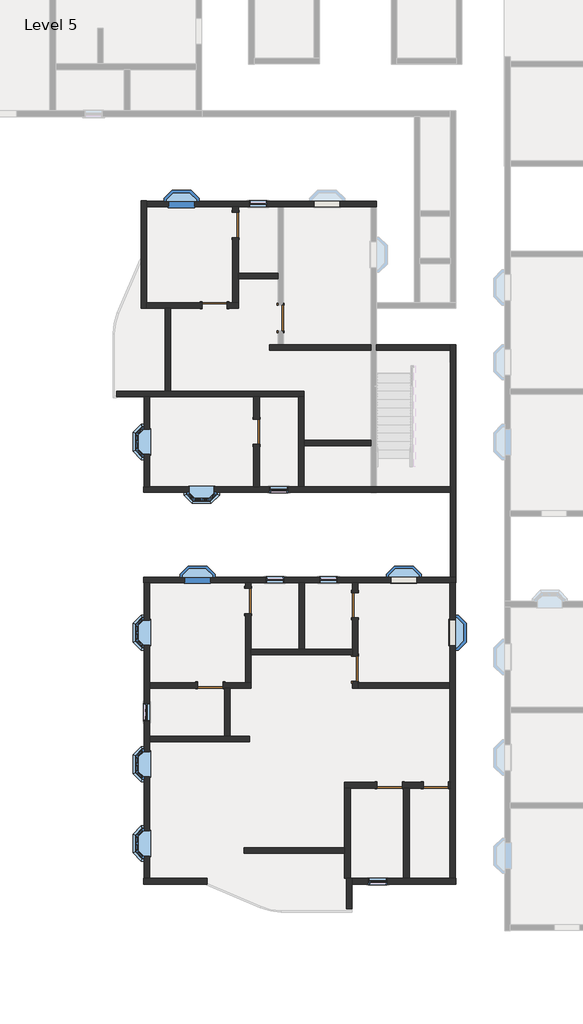
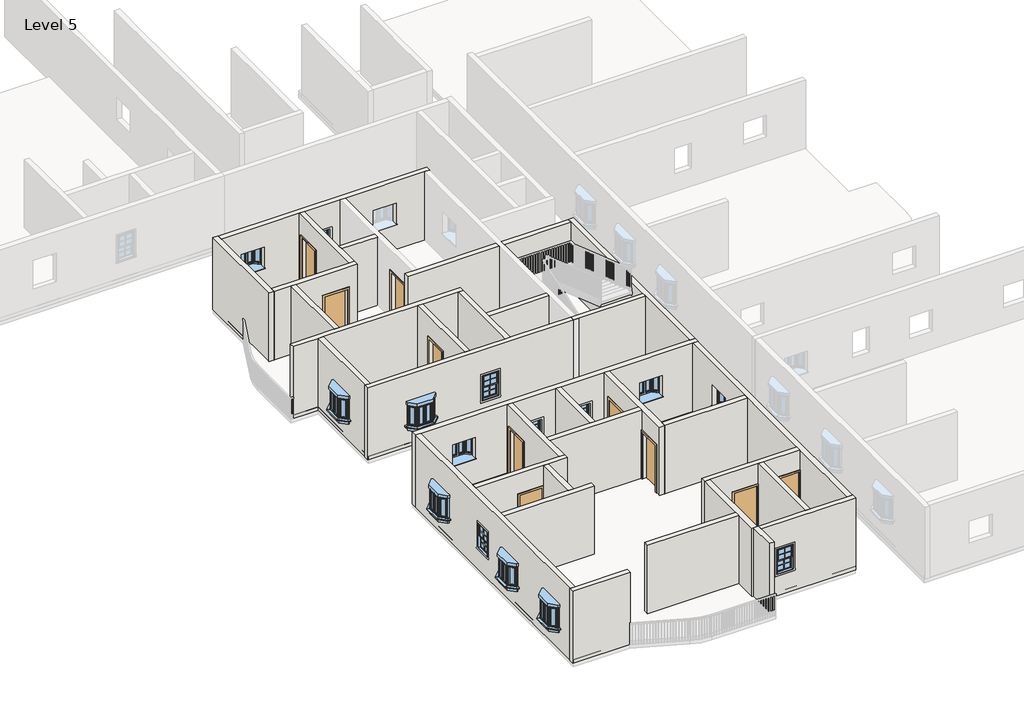
# One storey, part 1 of 14: 32 walls, 15 windows, 10 doors.
"""IFC4 building model written with IfcOpenShell, lengths in millimetres."""

from ifc_helpers import new_model, si_unit, frame, origin, place, context, project, spatial, polyline, outline, extrude, faceted_brep, transform, mapped, element, save
from components import door_54dd4da4, door_719f80de, window_910x910mm_67ef725a, window_8debb0fa

model = new_model("IFC4")

# Units and contexts
model_context = context("Model", 3, world=origin())
ifc_project = project(units=[si_unit("LENGTHUNIT", "METRE", prefix="MILLI")], contexts=[model_context])

# Site, building, storey
site = spatial("IfcSite", under=ifc_project)
building = spatial("IfcBuilding", under=site)
storey = spatial("IfcBuildingStorey", under=building, Name="Level 5", Elevation=12192.0)

# Doors
placement = place(None, origin())
door_shape = door_54dd4da4(model_context)
element("IfcDoor", 1, ObjectType="Single-Flush : 36\" x 84\"", at=placement, inside=storey, context=model_context, shape_type="MappedRepresentation", body=[
    mapped(door_shape, transform((-4626.037215, -17283.4916506, 12192.0), x_axis=(0.0, -1.0, 0.0), y_axis=(1.0, 0.0, 0.0), z_axis=(0.0, 0.0, 1.0))),
])
element("IfcDoor", 2, ObjectType="Single-Flush : 36\" x 84\"", at=placement, inside=storey, context=model_context, shape_type="MappedRepresentation", body=[
    mapped(door_shape, transform((-4626.037215, -14978.4416506, 12192.0), x_axis=(0.0, 1.0, 0.0), y_axis=(-1.0, 0.0, 0.0), z_axis=(0.0, 0.0, 1.0))),
])
element("IfcDoor", 3, ObjectType="Single-Flush : 36\" x 84\"", at=placement, inside=storey, context=model_context, shape_type="MappedRepresentation", body=[
    mapped(door_shape, transform((-9731.437215, -4100.8916506, 12192.0), x_axis=(1.0, 0.0, 0.0), y_axis=(0.0, 1.0, 0.0), z_axis=(0.0, 0.0, 1.0))),
])
element("IfcDoor", 4, ObjectType="Single-Flush : 36\" x 84\"", at=placement, inside=storey, context=model_context, shape_type="MappedRepresentation", body=[
    mapped(door_shape, transform((-7331.137215, -4558.0916506, 12192.0), x_axis=(0.0, -1.0, 0.0), y_axis=(1.0, 0.0, 0.0), z_axis=(0.0, 0.0, 1.0))),
])
door_2_shape = door_719f80de(model_context)
element("IfcDoor", 5, ObjectType="Single-Flush : 36\" x 84\"", at=placement, inside=storey, context=model_context, shape_type="MappedRepresentation", body=[
    mapped(door_2_shape, transform((-9883.837215, -17891.2072331, 12192.0), x_axis=(1.0, 0.0, 0.0), y_axis=(0.0, 1.0, 0.0), z_axis=(0.0, 0.0, 1.0))),
])
element("IfcDoor", 6, ObjectType="Single-Flush : 36\" x 84\"", at=placement, inside=storey, context=model_context, shape_type="MappedRepresentation", body=[
    mapped(door_2_shape, transform((-8512.237215, -14826.0416506, 12192.0), x_axis=(0.0, 1.0, 0.0), y_axis=(-1.0, 0.0, 0.0), z_axis=(0.0, 0.0, 1.0))),
])
element("IfcDoor", 7, ObjectType="Single-Flush : 36\" x 84\"", at=placement, inside=storey, context=model_context, shape_type="MappedRepresentation", body=[
    mapped(door_2_shape, transform((-8207.437215, -8691.9416506, 12192.0), x_axis=(0.0, 1.0, 0.0), y_axis=(-1.0, 0.0, 0.0), z_axis=(0.0, 0.0, 1.0))),
])
element("IfcDoor", 8, ObjectType="Single-Flush : 36\" x 84\"", at=placement, inside=storey, context=model_context, shape_type="MappedRepresentation", body=[
    mapped(door_2_shape, transform((-8969.437215, -1186.2416506, 12192.0), x_axis=(0.0, 1.0, 0.0), y_axis=(-1.0, 0.0, 0.0), z_axis=(0.0, 0.0, 1.0))),
])
element("IfcDoor", 9, ObjectType="Single-Flush : 36\" x 84\"", at=placement, inside=storey, context=model_context, shape_type="MappedRepresentation", body=[
    mapped(door_2_shape, transform((-3374.4891351, -21512.5916506, 12192.0), x_axis=(1.0, 0.0, 0.0), y_axis=(0.0, 1.0, 0.0), z_axis=(0.0, 0.0, 1.0))),
])
element("IfcDoor", 10, ObjectType="Single-Flush : 36\" x 84\"", at=placement, inside=storey, context=model_context, shape_type="MappedRepresentation", body=[
    mapped(door_2_shape, transform((-1698.0891351, -21512.5916506, 12192.0), x_axis=(1.0, 0.0, 0.0), y_axis=(0.0, 1.0, 0.0), z_axis=(0.0, 0.0, 1.0))),
])

# Walls
element("IfcWall", 11, ObjectType="4.5\" p", at=placement, inside=storey, context=model_context, shape_type="Brep", body=[
    faceted_brep([(-9426.637215, -17992.8072331, 14325.6), (-9426.637215, -17992.8072331, 12192.0), (-9375.837215, -17992.8072331, 12192.0), (-9172.637215, -17992.8072331, 12192.0), (-8410.637215, -17992.8072331, 12192.0), (-8410.637215, -17992.8072331, 15240.0), (-9172.637215, -17992.8072331, 15240.0), (-9375.837215, -17992.8072331, 15240.0), (-12087.287215, -17992.8072331, 15240.0), (-12087.287215, -17992.8072331, 12192.0), (-10341.037215, -17992.8072331, 12192.0), (-10341.037215, -17992.8072331, 14325.6), (-8410.637215, -17789.6072331, 12192.0), (-8613.837215, -17789.6072331, 12192.0), (-9426.637215, -17789.6072331, 12192.0), (-9426.637215, -17789.6072331, 14325.6), (-10341.037215, -17789.6072331, 14325.6), (-10341.037215, -17789.6072331, 12192.0), (-12087.287215, -17789.6072331, 12192.0), (-12087.287215, -17789.6072331, 15240.0), (-8613.837215, -17789.6072331, 15240.0), (-8410.637215, -17789.6072331, 15240.0)], [[[0, 1, 2, 3, 4, 5, 6, 7, 8, 9, 10, 11]], [[12, 13, 14, 15, 16, 17, 18, 19, 20, 21]], [[10, 9, 18, 17]], [[4, 3, 2, 1, 14, 13, 12]], [[8, 7, 6, 5, 21, 20, 19]], [[9, 8, 19, 18]], [[5, 4, 12, 21]], [[15, 14, 1, 0]], [[16, 15, 0, 11]], [[17, 16, 11, 10]]]),
])
element("IfcWall", 12, ObjectType="4.5\" p", at=placement, inside=storey, context=model_context, shape_type="Brep", body=[
    faceted_brep([(-8410.637215, -14368.8416506, 14325.6), (-8410.637215, -14368.8416506, 12192.0), (-8410.637215, -14165.6416506, 12192.0), (-8410.637215, -14165.6416506, 15240.0), (-8410.637215, -16572.2916506, 15240.0), (-8410.637215, -16775.4916506, 15240.0), (-8410.637215, -17789.6072331, 15240.0), (-8410.637215, -17789.6072331, 12192.0), (-8410.637215, -16775.4916506, 12192.0), (-8410.637215, -16572.2916506, 12192.0), (-8410.637215, -15283.2416506, 12192.0), (-8410.637215, -15283.2416506, 14325.6), (-8613.837215, -14165.6416506, 12192.0), (-8613.837215, -14368.8416506, 12192.0), (-8613.837215, -14368.8416506, 14325.6), (-8613.837215, -15283.2416506, 14325.6), (-8613.837215, -15283.2416506, 12192.0), (-8613.837215, -17789.6072331, 12192.0), (-8613.837215, -17789.6072331, 15240.0), (-8613.837215, -14165.6416506, 15240.0)], [[[0, 1, 2, 3, 4, 5, 6, 7, 8, 9, 10, 11]], [[12, 13, 14, 15, 16, 17, 18, 19]], [[2, 1, 13, 12]], [[10, 9, 8, 7, 17, 16]], [[6, 5, 4, 3, 19, 18]], [[7, 6, 18, 17]], [[3, 2, 12, 19]], [[14, 13, 1, 0]], [[15, 14, 0, 11]], [[16, 15, 11, 10]]]),
])
element("IfcWall", 13, ObjectType="4.5\" p", at=placement, inside=storey, context=model_context, shape_type="Brep", body=[
    faceted_brep([(-8410.637215, -16775.4916506, 12192.0), (-4727.637215, -16775.4916506, 12192.0), (-4727.637215, -16775.4916506, 15240.0), (-8410.637215, -16775.4916506, 15240.0), (-8410.637215, -16572.2916506, 12192.0), (-8410.637215, -16572.2916506, 15240.0), (-6670.737215, -16572.2916506, 15240.0), (-6467.537215, -16572.2916506, 15240.0), (-4727.637215, -16572.2916506, 15240.0), (-4727.637215, -16572.2916506, 12192.0), (-6467.537215, -16572.2916506, 12192.0), (-6670.737215, -16572.2916506, 12192.0)], [[[0, 1, 2, 3]], [[4, 5, 6, 7, 8, 9, 10, 11]], [[1, 0, 4, 11, 10, 9]], [[3, 2, 8, 7, 6, 5]], [[0, 3, 5, 4]], [[2, 1, 9, 8]]]),
])
element("IfcWall", 14, ObjectType="4.5\" p", at=placement, inside=storey, context=model_context, shape_type="SweptSolid", body=[
    extrude(outline(polyline([(-6670.737215, -16572.2916506), (-6670.737215, -14165.6416506), (-6467.537215, -14165.6416506), (-6467.537215, -16572.2916506), (-6670.737215, -16572.2916506)])), frame((0.0, 0.0, 12192.0), z_axis=(0.0, 0.0, 1.0), x_axis=(1.0, 0.0, 0.0)), (0.0, 0.0, 1.0), 3048.0),
])
element("IfcWall", 15, ObjectType="4.5\" p", at=placement, inside=storey, context=model_context, shape_type="Brep", body=[
    faceted_brep([(-4727.637215, -14165.6416506, 12192.0), (-4727.637215, -14521.2416506, 12192.0), (-4727.637215, -14521.2416506, 14325.6), (-4727.637215, -15435.6416506, 14325.6), (-4727.637215, -15435.6416506, 12192.0), (-4727.637215, -16572.2916506, 12192.0), (-4727.637215, -16775.4916506, 12192.0), (-4727.637215, -16826.2916506, 12192.0), (-4727.637215, -16826.2916506, 14325.6), (-4727.637215, -17740.6916506, 14325.6), (-4727.637215, -17740.6916506, 12192.0), (-4727.637215, -17994.6916506, 12192.0), (-4727.637215, -17994.6916506, 15240.0), (-4727.637215, -16775.4916506, 15240.0), (-4727.637215, -16572.2916506, 15240.0), (-4727.637215, -14165.6416506, 15240.0), (-4524.437215, -14521.2416506, 14325.6), (-4524.437215, -14521.2416506, 12192.0), (-4524.437215, -14165.6416506, 12192.0), (-4524.437215, -14165.6416506, 15240.0), (-4524.437215, -17791.4916506, 15240.0), (-4524.437215, -17994.6916506, 15240.0), (-4524.437215, -17994.6916506, 12192.0), (-4524.437215, -17791.4916506, 12192.0), (-4524.437215, -17740.6916506, 12192.0), (-4524.437215, -17740.6916506, 14325.6), (-4524.437215, -16826.2916506, 14325.6), (-4524.437215, -16826.2916506, 12192.0), (-4524.437215, -15435.6416506, 12192.0), (-4524.437215, -15435.6416506, 14325.6)], [[[0, 1, 2, 3, 4, 5, 6, 7, 8, 9, 10, 11, 12, 13, 14, 15]], [[16, 17, 18, 19, 20, 21, 22, 23, 24, 25, 26, 27, 28, 29]], [[11, 10, 24, 23, 22]], [[28, 27, 7, 6, 5, 4]], [[18, 17, 1, 0]], [[15, 14, 13, 12, 21, 20, 19]], [[0, 15, 19, 18]], [[12, 11, 22, 21]], [[25, 24, 10, 9]], [[26, 25, 9, 8]], [[27, 26, 8, 7]], [[2, 1, 17, 16]], [[3, 2, 16, 29]], [[4, 3, 29, 28]]]),
])
element("IfcWall", 16, ObjectType="4.5\" p", at=placement, inside=storey, context=model_context, shape_type="SweptSolid", body=[
    extrude(outline(polyline([(-4524.437215, -17791.4916506), (-1190.0891351, -17791.4916506), (-1190.0891351, -17994.6916506), (-4524.437215, -17994.6916506), (-4524.437215, -17791.4916506)])), frame((0.0, 0.0, 12192.0), z_axis=(0.0, 0.0, 1.0), x_axis=(1.0, 0.0, 0.0)), (0.0, 0.0, 1.0), 3048.0),
])
element("IfcWall", 17, ObjectType="4.5\" p", at=placement, inside=storey, context=model_context, shape_type="SweptSolid", body=[
    extrude(outline(polyline([(-9375.837215, -19734.5916506), (-9375.837215, -17992.8072331), (-9172.637215, -17992.8072331), (-9172.637215, -19734.5916506), (-9375.837215, -19734.5916506)])), frame((0.0, 0.0, 12192.0), z_axis=(0.0, 0.0, 1.0), x_axis=(1.0, 0.0, 0.0)), (0.0, 0.0, 1.0), 3048.0),
])
element("IfcWall", 18, ObjectType="4.5\" p", at=placement, inside=storey, context=model_context, shape_type="Brep", body=[
    faceted_brep([(-12087.287215, -19937.7916506, 12192.0), (-8455.087215, -19937.7916506, 12192.0), (-8455.087215, -19937.7916506, 15240.0), (-12087.287215, -19937.7916506, 15240.0), (-12087.287215, -19734.5916506, 12192.0), (-12087.287215, -19734.5916506, 15240.0), (-9375.837215, -19734.5916506, 15240.0), (-9172.637215, -19734.5916506, 15240.0), (-8455.087215, -19734.5916506, 15240.0), (-8455.087215, -19734.5916506, 12192.0), (-9172.637215, -19734.5916506, 12192.0), (-9375.837215, -19734.5916506, 12192.0)], [[[0, 1, 2, 3]], [[4, 5, 6, 7, 8, 9, 10, 11]], [[1, 0, 4, 11, 10, 9]], [[2, 1, 9, 8]], [[3, 2, 8, 7, 6, 5]], [[0, 3, 5, 4]]]),
])
element("IfcWall", 19, ObjectType="4.5\" p", at=placement, inside=storey, context=model_context, shape_type="Brep", body=[
    faceted_brep([(-13293.787215, -7421.9416506, 12192.0), (-12290.487215, -7421.9416506, 12192.0), (-12087.287215, -7421.9416506, 12192.0), (-8309.037215, -7421.9416506, 12192.0), (-8105.837215, -7421.9416506, 12192.0), (-6689.787215, -7421.9416506, 12192.0), (-6486.587215, -7421.9416506, 12192.0), (-6486.587215, -7421.9416506, 15240.0), (-6689.787215, -7421.9416506, 15240.0), (-8105.837215, -7421.9416506, 15240.0), (-8309.037215, -7421.9416506, 15240.0), (-12087.287215, -7421.9416506, 15240.0), (-12290.487215, -7421.9416506, 15240.0), (-13293.787215, -7421.9416506, 15240.0), (-13293.787215, -7218.7416506, 12192.0), (-13293.787215, -7218.7416506, 15240.0), (-11528.487215, -7218.7416506, 15240.0), (-11325.287215, -7218.7416506, 15240.0), (-6486.587215, -7218.7416506, 15240.0), (-6486.587215, -7218.7416506, 12192.0), (-11325.287215, -7218.7416506, 12192.0), (-11528.487215, -7218.7416506, 12192.0)], [[[0, 1, 2, 3, 4, 5, 6, 7, 8, 9, 10, 11, 12, 13]], [[14, 15, 16, 17, 18, 19, 20, 21]], [[6, 5, 4, 3, 2, 1, 0, 14, 21, 20, 19]], [[13, 12, 11, 10, 9, 8, 7, 18, 17, 16, 15]], [[0, 13, 15, 14]], [[7, 6, 19, 18]]]),
])
element("IfcWall", 20, ObjectType="4.5\" p", at=placement, inside=storey, context=model_context, shape_type="Brep", body=[
    faceted_brep([(-12201.587215, -4202.4916506, 12192.0), (-12201.587215, -3999.2916506, 12192.0), (-12201.587215, -525.8416506, 12192.0), (-12201.587215, -322.6416506, 12192.0), (-12201.587215, -309.9416506, 12192.0), (-12201.587215, -309.9416506, 15240.0), (-12201.587215, -322.6416506, 15240.0), (-12201.587215, -525.8416506, 15240.0), (-12201.587215, -3999.2916506, 15240.0), (-12201.587215, -4202.4916506, 15240.0), (-12404.787215, -4202.4916506, 12192.0), (-12404.787215, -4202.4916506, 15240.0), (-12404.787215, -309.9416506, 15240.0), (-12404.787215, -309.9416506, 12192.0)], [[[0, 1, 2, 3, 4, 5, 6, 7, 8, 9]], [[10, 11, 12, 13]], [[4, 3, 2, 1, 0, 10, 13]], [[5, 4, 13, 12]], [[9, 8, 7, 6, 5, 12, 11]], [[0, 9, 11, 10]]]),
])
element("IfcWall", 21, ObjectType="4.5\" p", at=placement, inside=storey, context=model_context, shape_type="Brep", body=[
    faceted_brep([(-9274.237215, -4202.4916506, 14325.6), (-9274.237215, -4202.4916506, 12192.0), (-8867.837215, -4202.4916506, 12192.0), (-8867.837215, -4202.4916506, 15240.0), (-11325.287215, -4202.4916506, 15240.0), (-11528.487215, -4202.4916506, 15240.0), (-12201.587215, -4202.4916506, 15240.0), (-12201.587215, -4202.4916506, 12192.0), (-11528.487215, -4202.4916506, 12192.0), (-11325.287215, -4202.4916506, 12192.0), (-10188.637215, -4202.4916506, 12192.0), (-10188.637215, -4202.4916506, 14325.6), (-8867.837215, -3999.2916506, 12192.0), (-9071.037215, -3999.2916506, 12192.0), (-9274.237215, -3999.2916506, 12192.0), (-9274.237215, -3999.2916506, 14325.6), (-10188.637215, -3999.2916506, 14325.6), (-10188.637215, -3999.2916506, 12192.0), (-12201.587215, -3999.2916506, 12192.0), (-12201.587215, -3999.2916506, 15240.0), (-9071.037215, -3999.2916506, 15240.0), (-8867.837215, -3999.2916506, 15240.0)], [[[0, 1, 2, 3, 4, 5, 6, 7, 8, 9, 10, 11]], [[12, 13, 14, 15, 16, 17, 18, 19, 20, 21]], [[2, 1, 14, 13, 12]], [[10, 9, 8, 7, 18, 17]], [[6, 5, 4, 3, 21, 20, 19]], [[7, 6, 19, 18]], [[3, 2, 12, 21]], [[15, 14, 1, 0]], [[16, 15, 0, 11]], [[17, 16, 11, 10]]]),
])
element("IfcWall", 22, ObjectType="4.5\" p", at=placement, inside=storey, context=model_context, shape_type="Brep", body=[
    faceted_brep([(-8867.837215, -729.0416506, 14325.6), (-8867.837215, -729.0416506, 12192.0), (-8867.837215, -525.8416506, 12192.0), (-8867.837215, -525.8416506, 15240.0), (-8867.837215, -2932.4916506, 15240.0), (-8867.837215, -3135.6916506, 15240.0), (-8867.837215, -3999.2916506, 15240.0), (-8867.837215, -3999.2916506, 12192.0), (-8867.837215, -3135.6916506, 12192.0), (-8867.837215, -2932.4916506, 12192.0), (-8867.837215, -1643.4416506, 12192.0), (-8867.837215, -1643.4416506, 14325.6), (-9071.037215, -525.8416506, 12192.0), (-9071.037215, -729.0416506, 12192.0), (-9071.037215, -729.0416506, 14325.6), (-9071.037215, -1643.4416506, 14325.6), (-9071.037215, -1643.4416506, 12192.0), (-9071.037215, -3999.2916506, 12192.0), (-9071.037215, -3999.2916506, 15240.0), (-9071.037215, -525.8416506, 15240.0)], [[[0, 1, 2, 3, 4, 5, 6, 7, 8, 9, 10, 11]], [[12, 13, 14, 15, 16, 17, 18, 19]], [[2, 1, 13, 12]], [[10, 9, 8, 7, 17, 16]], [[6, 5, 4, 3, 19, 18]], [[7, 6, 18, 17]], [[3, 2, 12, 19]], [[14, 13, 1, 0]], [[15, 14, 0, 11]], [[16, 15, 11, 10]]]),
])
element("IfcWall", 23, ObjectType="4.5\" p", at=placement, inside=storey, context=model_context, shape_type="SweptSolid", body=[
    extrude(outline(polyline([(-7432.737215, -3135.6916506), (-8867.837215, -3135.6916506), (-8867.837215, -2932.4916506), (-7432.737215, -2932.4916506), (-7432.737215, -3135.6916506)])), frame((0.0, 0.0, 12192.0), z_axis=(0.0, 0.0, 1.0), x_axis=(1.0, 0.0, 0.0)), (0.0, 0.0, 1.0), 3048.0),
])
element("IfcWall", 24, ObjectType="4.5\" p", at=placement, inside=storey, context=model_context, shape_type="Brep", body=[
    faceted_brep([(-7731.187215, -5726.4916506, 15240.0), (-7731.187215, -5726.4916506, 12192.0), (-4060.887215, -5726.4916506, 12192.0), (-4060.887215, -5726.4916506, 15240.0), (-7731.187215, -5523.2916506, 12192.0), (-7731.187215, -5523.2916506, 15240.0), (-7432.737215, -5523.2916506, 15240.0), (-7229.537215, -5523.2916506, 15240.0), (-4060.887215, -5523.2916506, 15240.0), (-4060.887215, -5523.2916506, 12192.0), (-7229.537215, -5523.2916506, 12192.0), (-7432.737215, -5523.2916506, 12192.0)], [[[0, 1, 2, 3]], [[4, 5, 6, 7, 8, 9, 10, 11]], [[1, 4, 11, 10, 9, 2]], [[5, 0, 3, 8, 7, 6]], [[1, 0, 5, 4]], [[3, 2, 9, 8]]]),
    faceted_brep([(-1177.3891351, -5726.4916506, 12192.0), (-1177.3891351, -5726.4916506, 15240.0), (-3857.687215, -5726.4916506, 15240.0), (-3857.687215, -5726.4916506, 12192.0), (-1177.3891351, -5523.2916506, 15240.0), (-1177.3891351, -5523.2916506, 12192.0), (-3857.687215, -5523.2916506, 12192.0), (-3857.687215, -5523.2916506, 15240.0)], [[[0, 1, 2, 3]], [[4, 5, 6, 7]], [[5, 0, 3, 6]], [[1, 4, 7, 2]], [[1, 0, 5, 4]], [[3, 2, 7, 6]]]),
])
element("IfcWall", 25, ObjectType="4.5\" p", at=placement, inside=storey, context=model_context, shape_type="SweptSolid", body=[
    extrude(outline(polyline([(-11528.487215, -7218.7416506), (-11528.487215, -4202.4916506), (-11325.287215, -4202.4916506), (-11325.287215, -7218.7416506), (-11528.487215, -7218.7416506)])), frame((0.0, 0.0, 12192.0), z_axis=(0.0, 0.0, 1.0), x_axis=(1.0, 0.0, 0.0)), (0.0, 0.0, 1.0), 3048.0),
])
element("IfcWall", 26, ObjectType="4.5\" p", at=placement, inside=storey, context=model_context, shape_type="SweptSolid", body=[
    extrude(outline(polyline([(-7421.9416506, 12192.0), (-8234.7416506, 12192.0), (-8234.7416506, 14325.6), (-9149.1416506, 14325.6), (-9149.1416506, 12192.0), (-10685.8416506, 12192.0), (-10685.8416506, 15240.0), (-7421.9416506, 15240.0), (-7421.9416506, 12192.0)])), frame((-8309.037215, 0.0, 0.0), z_axis=(1.0, 0.0, 0.0), x_axis=(0.0, 1.0, 0.0)), (0.0, 0.0, 1.0), 203.2),
])
element("IfcWall", 27, ObjectType="4.5\" p", at=placement, inside=storey, context=model_context, shape_type="Brep", body=[
    faceted_brep([(-6689.787215, -7421.9416506, 12192.0), (-6689.787215, -10685.8416506, 12192.0), (-6689.787215, -10685.8416506, 15240.0), (-6689.787215, -7421.9416506, 15240.0), (-6486.587215, -7421.9416506, 12192.0), (-6486.587215, -7421.9416506, 15240.0), (-6486.587215, -8990.3916506, 15240.0), (-6486.587215, -9193.5916506, 15240.0), (-6486.587215, -10685.8416506, 15240.0), (-6486.587215, -10685.8416506, 12192.0), (-6486.587215, -9193.5916506, 12192.0), (-6486.587215, -8990.3916506, 12192.0)], [[[0, 1, 2, 3]], [[4, 5, 6, 7, 8, 9, 10, 11]], [[1, 0, 4, 11, 10, 9]], [[3, 2, 8, 7, 6, 5]], [[0, 3, 5, 4]], [[2, 1, 9, 8]]]),
])
element("IfcWall", 28, ObjectType="4.5\" p", at=placement, inside=storey, context=model_context, shape_type="SweptSolid", body=[
    extrude(outline(polyline([(-4060.887215, -9193.5916506), (-6486.587215, -9193.5916506), (-6486.587215, -8990.3916506), (-4060.887215, -8990.3916506), (-4060.887215, -9193.5916506)])), frame((0.0, 0.0, 12192.0), z_axis=(0.0, 0.0, 1.0), x_axis=(1.0, 0.0, 0.0)), (0.0, 0.0, 1.0), 3048.0),
])
element("IfcWall", 29, ObjectType="9\"", at=placement, inside=storey, context=model_context, shape_type="Brep", body=[
    faceted_brep([(-1190.0891351, -21410.9916506, 12192.0), (-1240.8891351, -21410.9916506, 12192.0), (-1240.8891351, -21410.9916506, 14325.6), (-2155.2891351, -21410.9916506, 14325.6), (-2155.2891351, -21410.9916506, 12192.0), (-2917.2891351, -21410.9916506, 12192.0), (-2917.2891351, -21410.9916506, 14325.6), (-3831.6891351, -21410.9916506, 14325.6), (-3831.6891351, -21410.9916506, 12192.0), (-5006.4391351, -21410.9916506, 12192.0), (-5006.4391351, -21410.9916506, 15240.0), (-1190.0891351, -21410.9916506, 15240.0), (-1240.8891351, -21614.1916506, 14325.6), (-1240.8891351, -21614.1916506, 12192.0), (-1190.0891351, -21614.1916506, 12192.0), (-1190.0891351, -21614.1916506, 15240.0), (-2663.2891351, -21614.1916506, 15240.0), (-2866.4891351, -21614.1916506, 15240.0), (-4803.2391351, -21614.1916506, 15240.0), (-5006.4391351, -21614.1916506, 15240.0), (-5006.4391351, -21614.1916506, 12192.0), (-4803.2391351, -21614.1916506, 12192.0), (-3831.6891351, -21614.1916506, 12192.0), (-3831.6891351, -21614.1916506, 14325.6), (-2917.2891351, -21614.1916506, 14325.6), (-2917.2891351, -21614.1916506, 12192.0), (-2866.4891351, -21614.1916506, 12192.0), (-2663.2891351, -21614.1916506, 12192.0), (-2155.2891351, -21614.1916506, 12192.0), (-2155.2891351, -21614.1916506, 14325.6)], [[[0, 1, 2, 3, 4, 5, 6, 7, 8, 9, 10, 11]], [[12, 13, 14, 15, 16, 17, 18, 19, 20, 21, 22, 23, 24, 25, 26, 27, 28, 29]], [[22, 21, 20, 9, 8]], [[14, 13, 1, 0]], [[28, 27, 26, 25, 5, 4]], [[11, 10, 19, 18, 17, 16, 15]], [[0, 11, 15, 14]], [[10, 9, 20, 19]], [[6, 5, 25, 24]], [[7, 6, 24, 23]], [[8, 7, 23, 22]], [[2, 1, 13, 12]], [[3, 2, 12, 29]], [[4, 3, 29, 28]]]),
])
element("IfcWall", 30, ObjectType="9\"", at=placement, inside=storey, context=model_context, shape_type="Brep", body=[
    faceted_brep([(-5006.4391351, -21614.1916506, 12192.0), (-5006.4391351, -23779.5416506, 12192.0), (-5006.4391351, -23982.7416506, 12192.0), (-5006.4391351, -24897.1416506, 12192.0), (-5006.4391351, -24897.1416506, 15240.0), (-5006.4391351, -23982.7416506, 15240.0), (-5006.4391351, -23779.5416506, 15240.0), (-5006.4391351, -21614.1916506, 15240.0), (-4803.2391351, -21614.1916506, 12192.0), (-4803.2391351, -21614.1916506, 15240.0), (-4803.2391351, -24897.1416506, 15240.0), (-4803.2391351, -24897.1416506, 12192.0), (-4949.2891351, -24897.1416506, 12192.0), (-4949.2891351, -24897.1416506, 15240.0)], [[[0, 1, 2, 3, 4, 5, 6, 7]], [[8, 9, 10, 11]], [[3, 2, 1, 0, 8, 11, 12]], [[7, 6, 5, 4, 13, 10, 9]], [[0, 7, 9, 8]], [[4, 3, 12, 11, 10, 13]]]),
])
element("IfcWall", 31, ObjectType="9\"", at=placement, inside=storey, context=model_context, shape_type="SweptSolid", body=[
    extrude(outline(polyline([(-2866.4891351, -24897.1416506), (-2866.4891351, -21614.1916506), (-2663.2891351, -21614.1916506), (-2663.2891351, -24897.1416506), (-2866.4891351, -24897.1416506)])), frame((0.0, 0.0, 12192.0), z_axis=(0.0, 0.0, 1.0), x_axis=(1.0, 0.0, 0.0)), (0.0, 0.0, 1.0), 3048.0),
])
element("IfcWall", 32, ObjectType="9\"", at=placement, inside=storey, context=model_context, shape_type="SweptSolid", body=[
    extrude(outline(polyline([(-5006.4391351, -23982.7416506), (-8664.637215, -23982.7416506), (-8664.637215, -23779.5416506), (-5006.4391351, -23779.5416506), (-5006.4391351, -23982.7416506)])), frame((0.0, 0.0, 12192.0), z_axis=(0.0, 0.0, 1.0), x_axis=(1.0, 0.0, 0.0)), (0.0, 0.0, 1.0), 3048.0),
])
element("IfcWall", 33, ObjectType="9\" w", at=placement, inside=storey, context=model_context, shape_type="Brep", body=[
    faceted_brep([(-12303.187215, -14165.6416506, 12192.0), (-12290.487215, -14165.6416506, 12192.0), (-12087.287215, -14165.6416506, 12192.0), (-8613.837215, -14165.6416506, 12192.0), (-8410.637215, -14165.6416506, 12192.0), (-6670.737215, -14165.6416506, 12192.0), (-6467.537215, -14165.6416506, 12192.0), (-4727.637215, -14165.6416506, 12192.0), (-4524.437215, -14165.6416506, 12192.0), (-1190.0891351, -14165.6416506, 12192.0), (-986.8891351, -14165.6416506, 12192.0), (-961.4891351, -14165.6416506, 12192.0), (-961.4891351, -14165.6416506, 15240.0), (-986.8891351, -14165.6416506, 15240.0), (-1190.0891351, -14165.6416506, 15240.0), (-4524.437215, -14165.6416506, 15240.0), (-4727.637215, -14165.6416506, 15240.0), (-6467.537215, -14165.6416506, 15240.0), (-6670.737215, -14165.6416506, 15240.0), (-8410.637215, -14165.6416506, 15240.0), (-8613.837215, -14165.6416506, 15240.0), (-12087.287215, -14165.6416506, 15240.0), (-12290.487215, -14165.6416506, 15240.0), (-12303.187215, -14165.6416506, 15240.0), (-10805.562215, -14165.6416506, 14302.0), (-9895.562215, -14165.6416506, 14302.0), (-9895.562215, -14165.6416506, 13392.0), (-10805.562215, -14165.6416506, 13392.0), (-3312.2631751, -14165.6416506, 14302.0), (-2402.2631751, -14165.6416506, 14302.0), (-2402.2631751, -14165.6416506, 13392.0), (-3312.2631751, -14165.6416506, 13392.0), (-7870.887215, -14165.6416506, 14173.2), (-7210.487215, -14165.6416506, 14173.2), (-7210.487215, -14165.6416506, 13106.4), (-7870.887215, -14165.6416506, 13106.4), (-5927.787215, -14165.6416506, 14173.2), (-5267.387215, -14165.6416506, 14173.2), (-5267.387215, -14165.6416506, 13106.4), (-5927.787215, -14165.6416506, 13106.4), (-12303.187215, -13962.4416506, 12192.0), (-12303.187215, -13962.4416506, 15240.0), (-1177.3891351, -13962.4416506, 15240.0), (-974.1891351, -13962.4416506, 15240.0), (-961.4891351, -13962.4416506, 15240.0), (-961.4891351, -13962.4416506, 12192.0), (-974.1891351, -13962.4416506, 12192.0), (-1177.3891351, -13962.4416506, 12192.0), (-10805.562215, -13962.4416506, 14302.0), (-10805.562215, -13962.4416506, 13392.0), (-9895.562215, -13962.4416506, 13392.0), (-9895.562215, -13962.4416506, 14302.0), (-3312.2631751, -13962.4416506, 14302.0), (-3312.2631751, -13962.4416506, 13392.0), (-2402.2631751, -13962.4416506, 13392.0), (-2402.2631751, -13962.4416506, 14302.0), (-7870.887215, -13962.4416506, 14173.2), (-7870.887215, -13962.4416506, 13106.4), (-7210.487215, -13962.4416506, 13106.4), (-7210.487215, -13962.4416506, 14173.2), (-5927.787215, -13962.4416506, 14173.2), (-5927.787215, -13962.4416506, 13106.4), (-5267.387215, -13962.4416506, 13106.4), (-5267.387215, -13962.4416506, 14173.2)], [[[0, 1, 2, 3, 4, 5, 6, 7, 8, 9, 10, 11, 12, 13, 14, 15, 16, 17, 18, 19, 20, 21, 22, 23], [24, 25, 26, 27], [28, 29, 30, 31], [32, 33, 34, 35], [36, 37, 38, 39]], [[40, 41, 42, 43, 44, 45, 46, 47], [48, 49, 50, 51], [52, 53, 54, 55], [56, 57, 58, 59], [60, 61, 62, 63]], [[11, 10, 9, 8, 7, 6, 5, 4, 3, 2, 1, 0, 40, 47, 46, 45]], [[12, 11, 45, 44]], [[23, 22, 21, 20, 19, 18, 17, 16, 15, 14, 13, 12, 44, 43, 42, 41]], [[0, 23, 41, 40]], [[49, 48, 24, 27]], [[50, 49, 27, 26]], [[51, 50, 26, 25]], [[48, 51, 25, 24]], [[53, 52, 28, 31]], [[54, 53, 31, 30]], [[55, 54, 30, 29]], [[52, 55, 29, 28]], [[57, 56, 32, 35]], [[58, 57, 35, 34]], [[59, 58, 34, 33]], [[56, 59, 33, 32]], [[61, 60, 36, 39]], [[62, 61, 39, 38]], [[63, 62, 38, 37]], [[60, 63, 37, 36]]]),
])
element("IfcWall", 34, ObjectType="9\" w", at=placement, inside=storey, context=model_context, shape_type="Brep", body=[
    faceted_brep([(-10004.0323936, -24897.1416506, 12192.0), (-12087.287215, -24897.1416506, 12192.0), (-12290.487215, -24897.1416506, 12192.0), (-12303.187215, -24897.1416506, 12192.0), (-12303.187215, -24897.1416506, 15240.0), (-12290.487215, -24897.1416506, 15240.0), (-12087.287215, -24897.1416506, 15240.0), (-10004.0323936, -24897.1416506, 15240.0), (-10004.0323936, -25100.3416506, 12192.0), (-10004.0323936, -25100.3416506, 15240.0), (-12303.187215, -25100.3416506, 15240.0), (-12303.187215, -25100.3416506, 12192.0)], [[[0, 1, 2, 3, 4, 5, 6, 7]], [[8, 9, 10, 11]], [[3, 2, 1, 0, 8, 11]], [[4, 3, 11, 10]], [[7, 6, 5, 4, 10, 9]], [[0, 7, 9, 8]]]),
])
element("IfcWall", 35, ObjectType="9\" w", at=placement, inside=storey, context=model_context, shape_type="Brep", body=[
    faceted_brep([(-4746.0891351, -25989.3416506, 12192.0), (-4746.0891351, -25100.3416506, 12192.0), (-4746.0891351, -24897.1416506, 12192.0), (-4746.0891351, -24897.1416506, 15240.0), (-4746.0891351, -25100.3416506, 15240.0), (-4746.0891351, -25989.3416506, 15240.0), (-4949.2891351, -25989.3416506, 12192.0), (-4949.2891351, -25989.3416506, 15240.0), (-4949.2891351, -24897.1416506, 15240.0), (-4949.2891351, -24897.1416506, 12192.0), (-4803.2391351, -24897.1416506, 12192.0), (-4803.2391351, -24897.1416506, 15240.0)], [[[0, 1, 2, 3, 4, 5]], [[6, 7, 8, 9]], [[2, 1, 0, 6, 9, 10]], [[5, 4, 3, 11, 8, 7]], [[0, 5, 7, 6]], [[3, 2, 10, 9, 8, 11]]]),
])
element("IfcWall", 36, ObjectType="9\" w", at=placement, inside=storey, context=model_context, shape_type="Brep", body=[
    faceted_brep([(-4746.0891351, -25100.3416506, 12192.0), (-961.4891351, -25100.3416506, 12192.0), (-961.4891351, -25100.3416506, 15240.0), (-4746.0891351, -25100.3416506, 15240.0), (-3476.0891351, -25100.3416506, 14173.2), (-3476.0891351, -25100.3416506, 13106.4), (-4136.4891351, -25100.3416506, 13106.4), (-4136.4891351, -25100.3416506, 14173.2), (-4746.0891351, -24897.1416506, 12192.0), (-4746.0891351, -24897.1416506, 15240.0), (-2866.4891351, -24897.1416506, 15240.0), (-2663.2891351, -24897.1416506, 15240.0), (-1190.0891351, -24897.1416506, 15240.0), (-986.8891351, -24897.1416506, 15240.0), (-961.4891351, -24897.1416506, 15240.0), (-961.4891351, -24897.1416506, 12192.0), (-986.8891351, -24897.1416506, 12192.0), (-1190.0891351, -24897.1416506, 12192.0), (-2663.2891351, -24897.1416506, 12192.0), (-2866.4891351, -24897.1416506, 12192.0), (-3476.0891351, -24897.1416506, 14173.2), (-4136.4891351, -24897.1416506, 14173.2), (-4136.4891351, -24897.1416506, 13106.4), (-3476.0891351, -24897.1416506, 13106.4)], [[[0, 1, 2, 3], [4, 5, 6, 7]], [[8, 9, 10, 11, 12, 13, 14, 15, 16, 17, 18, 19], [20, 21, 22, 23]], [[1, 0, 8, 19, 18, 17, 16, 15]], [[2, 1, 15, 14]], [[3, 2, 14, 13, 12, 11, 10, 9]], [[0, 3, 9, 8]], [[5, 4, 20, 23]], [[6, 5, 23, 22]], [[7, 6, 22, 21]], [[4, 7, 21, 20]]]),
])
element("IfcWall", 37, ObjectType="9\" w", at=placement, inside=storey, context=model_context, shape_type="Brep", body=[
    faceted_brep([(-12290.487215, -14165.6416506, 12192.0), (-12290.487215, -24897.1416506, 12192.0), (-12290.487215, -24897.1416506, 15240.0), (-12290.487215, -14165.6416506, 15240.0), (-12290.487215, -16432.6244419, 14016.4), (-12290.487215, -16432.6244419, 13106.4), (-12290.487215, -15522.6244419, 13106.4), (-12290.487215, -15522.6244419, 14016.4), (-12290.487215, -21205.5916506, 14016.4), (-12290.487215, -21205.5916506, 13106.4), (-12290.487215, -20295.5916506, 13106.4), (-12290.487215, -20295.5916506, 14016.4), (-12290.487215, -24082.1416506, 14016.4), (-12290.487215, -24082.1416506, 13106.4), (-12290.487215, -23172.1416506, 13106.4), (-12290.487215, -23172.1416506, 14016.4), (-12290.487215, -19193.8994419, 14173.2), (-12290.487215, -19193.8994419, 13106.4), (-12290.487215, -18533.4994419, 13106.4), (-12290.487215, -18533.4994419, 14173.2), (-12087.287215, -14165.6416506, 12192.0), (-12087.287215, -14165.6416506, 15240.0), (-12087.287215, -17789.6072331, 15240.0), (-12087.287215, -17992.8072331, 15240.0), (-12087.287215, -19734.5916506, 15240.0), (-12087.287215, -19937.7916506, 15240.0), (-12087.287215, -24897.1416506, 15240.0), (-12087.287215, -24897.1416506, 12192.0), (-12087.287215, -19937.7916506, 12192.0), (-12087.287215, -19734.5916506, 12192.0), (-12087.287215, -17992.8072331, 12192.0), (-12087.287215, -17789.6072331, 12192.0), (-12087.287215, -16432.6244419, 14016.4), (-12087.287215, -15522.6244419, 14016.4), (-12087.287215, -15522.6244419, 13106.4), (-12087.287215, -16432.6244419, 13106.4), (-12087.287215, -21205.5916506, 14016.4), (-12087.287215, -20295.5916506, 14016.4), (-12087.287215, -20295.5916506, 13106.4), (-12087.287215, -21205.5916506, 13106.4), (-12087.287215, -24082.1416506, 14016.4), (-12087.287215, -23172.1416506, 14016.4), (-12087.287215, -23172.1416506, 13106.4), (-12087.287215, -24082.1416506, 13106.4), (-12087.287215, -19193.8994419, 14173.2), (-12087.287215, -18533.4994419, 14173.2), (-12087.287215, -18533.4994419, 13106.4), (-12087.287215, -19193.8994419, 13106.4)], [[[0, 1, 2, 3], [4, 5, 6, 7], [8, 9, 10, 11], [12, 13, 14, 15], [16, 17, 18, 19]], [[20, 21, 22, 23, 24, 25, 26, 27, 28, 29, 30, 31], [32, 33, 34, 35], [36, 37, 38, 39], [40, 41, 42, 43], [44, 45, 46, 47]], [[1, 0, 20, 31, 30, 29, 28, 27]], [[3, 2, 26, 25, 24, 23, 22, 21]], [[0, 3, 21, 20]], [[2, 1, 27, 26]], [[5, 4, 32, 35]], [[6, 5, 35, 34]], [[7, 6, 34, 33]], [[4, 7, 33, 32]], [[9, 8, 36, 39]], [[10, 9, 39, 38]], [[11, 10, 38, 37]], [[8, 11, 37, 36]], [[13, 12, 40, 43]], [[14, 13, 43, 42]], [[15, 14, 42, 41]], [[12, 15, 41, 40]], [[17, 16, 44, 47]], [[18, 17, 47, 46]], [[19, 18, 46, 45]], [[16, 19, 45, 44]]]),
])
element("IfcWall", 38, ObjectType="9\" w", at=placement, inside=storey, context=model_context, shape_type="Brep", body=[
    faceted_brep([(-1190.0891351, -14165.6416506, 12192.0), (-1190.0891351, -17791.4916506, 12192.0), (-1190.0891351, -17994.6916506, 12192.0), (-1190.0891351, -21410.9916506, 12192.0), (-1190.0891351, -21614.1916506, 12192.0), (-1190.0891351, -24897.1416506, 12192.0), (-1190.0891351, -24897.1416506, 15240.0), (-1190.0891351, -21614.1916506, 15240.0), (-1190.0891351, -21410.9916506, 15240.0), (-1190.0891351, -17994.6916506, 15240.0), (-1190.0891351, -17791.4916506, 15240.0), (-1190.0891351, -14165.6416506, 15240.0), (-1190.0891351, -15523.5666506, 14302.0), (-1190.0891351, -16433.5666506, 14302.0), (-1190.0891351, -16433.5666506, 13392.0), (-1190.0891351, -15523.5666506, 13392.0), (-986.8891351, -14165.6416506, 12192.0), (-986.8891351, -14165.6416506, 15240.0), (-986.8891351, -24897.1416506, 15240.0), (-986.8891351, -24897.1416506, 12192.0), (-986.8891351, -15523.5666506, 14302.0), (-986.8891351, -15523.5666506, 13392.0), (-986.8891351, -16433.5666506, 13392.0), (-986.8891351, -16433.5666506, 14302.0)], [[[0, 1, 2, 3, 4, 5, 6, 7, 8, 9, 10, 11], [12, 13, 14, 15]], [[16, 17, 18, 19], [20, 21, 22, 23]], [[5, 4, 3, 2, 1, 0, 16, 19]], [[11, 10, 9, 8, 7, 6, 18, 17]], [[0, 11, 17, 16]], [[6, 5, 19, 18]], [[21, 20, 12, 15]], [[22, 21, 15, 14]], [[23, 22, 14, 13]], [[20, 23, 13, 12]]]),
])
element("IfcWall", 39, ObjectType="9\" w", at=placement, inside=storey, context=model_context, shape_type="Brep", body=[
    faceted_brep([(-1177.3891351, -5523.2916506, 12192.0), (-1177.3891351, -5726.4916506, 12192.0), (-1177.3891351, -10685.8416506, 12192.0), (-1177.3891351, -10889.0416506, 12192.0), (-1177.3891351, -13962.4416506, 12192.0), (-1177.3891351, -13962.4416506, 15240.0), (-1177.3891351, -10889.0416506, 15240.0), (-1177.3891351, -10685.8416506, 15240.0), (-1177.3891351, -5726.4916506, 15240.0), (-1177.3891351, -5523.2916506, 15240.0), (-974.1891351, -5523.2916506, 12192.0), (-974.1891351, -5523.2916506, 15240.0), (-974.1891351, -13962.4416506, 15240.0), (-974.1891351, -13962.4416506, 12192.0)], [[[0, 1, 2, 3, 4, 5, 6, 7, 8, 9]], [[10, 11, 12, 13]], [[4, 3, 2, 1, 0, 10, 13]], [[9, 8, 7, 6, 5, 12, 11]], [[5, 4, 13, 12]], [[0, 9, 11, 10]]]),
])
element("IfcWall", 40, ObjectType="9\" w", at=placement, inside=storey, context=model_context, shape_type="Brep", body=[
    faceted_brep([(-1177.3891351, -10685.8416506, 12192.0), (-6486.587215, -10685.8416506, 12192.0), (-6689.787215, -10685.8416506, 12192.0), (-8105.837215, -10685.8416506, 12192.0), (-8309.037215, -10685.8416506, 12192.0), (-12087.287215, -10685.8416506, 12192.0), (-12290.487215, -10685.8416506, 12192.0), (-12303.187215, -10685.8416506, 12192.0), (-12303.187215, -10685.8416506, 15240.0), (-12290.487215, -10685.8416506, 15240.0), (-12087.287215, -10685.8416506, 15240.0), (-8309.037215, -10685.8416506, 15240.0), (-8105.837215, -10685.8416506, 15240.0), (-6689.787215, -10685.8416506, 15240.0), (-6486.587215, -10685.8416506, 15240.0), (-1177.3891351, -10685.8416506, 15240.0), (-9743.162215, -10685.8416506, 14016.4), (-10653.162215, -10685.8416506, 14016.4), (-10653.162215, -10685.8416506, 13106.4), (-9743.162215, -10685.8416506, 13106.4), (-7067.612215, -10685.8416506, 14173.2), (-7728.012215, -10685.8416506, 14173.2), (-7728.012215, -10685.8416506, 13106.4), (-7067.612215, -10685.8416506, 13106.4), (-1177.3891351, -10889.0416506, 12192.0), (-1177.3891351, -10889.0416506, 15240.0), (-12303.187215, -10889.0416506, 15240.0), (-12303.187215, -10889.0416506, 12192.0), (-9743.162215, -10889.0416506, 14016.4), (-9743.162215, -10889.0416506, 13106.4), (-10653.162215, -10889.0416506, 13106.4), (-10653.162215, -10889.0416506, 14016.4), (-7067.612215, -10889.0416506, 14173.2), (-7067.612215, -10889.0416506, 13106.4), (-7728.012215, -10889.0416506, 13106.4), (-7728.012215, -10889.0416506, 14173.2)], [[[0, 1, 2, 3, 4, 5, 6, 7, 8, 9, 10, 11, 12, 13, 14, 15], [16, 17, 18, 19], [20, 21, 22, 23]], [[24, 25, 26, 27], [28, 29, 30, 31], [32, 33, 34, 35]], [[7, 6, 5, 4, 3, 2, 1, 0, 24, 27]], [[8, 7, 27, 26]], [[15, 14, 13, 12, 11, 10, 9, 8, 26, 25]], [[0, 15, 25, 24]], [[29, 28, 16, 19]], [[30, 29, 19, 18]], [[31, 30, 18, 17]], [[28, 31, 17, 16]], [[33, 32, 20, 23]], [[34, 33, 23, 22]], [[35, 34, 22, 21]], [[32, 35, 21, 20]]]),
])
element("IfcWall", 41, ObjectType="9\" w", at=placement, inside=storey, context=model_context, shape_type="SweptSolid", body=[
    extrude(outline(polyline([(-10685.8416506, 12192.0), (-10685.8416506, 15240.0), (-7421.9416506, 15240.0), (-7421.9416506, 12192.0), (-10685.8416506, 12192.0)]), holes=[polyline([(-9508.8916506, 14016.4), (-9508.8916506, 13106.4), (-8598.8916506, 13106.4), (-8598.8916506, 14016.4), (-9508.8916506, 14016.4)])]), frame((-12290.487215, 0.0, 0.0), z_axis=(1.0, 0.0, 0.0), x_axis=(0.0, 1.0, 0.0)), (0.0, 0.0, 1.0), 203.2),
])
element("IfcWall", 42, ObjectType="9\" w", at=placement, inside=storey, context=model_context, shape_type="Brep", body=[
    faceted_brep([(-12201.587215, -525.8416506, 12192.0), (-9071.037215, -525.8416506, 12192.0), (-8867.837215, -525.8416506, 12192.0), (-7432.737215, -525.8416506, 12192.0), (-7229.537215, -525.8416506, 12192.0), (-4060.887215, -525.8416506, 12192.0), (-3857.687215, -525.8416506, 12192.0), (-3844.987215, -525.8416506, 12192.0), (-3844.987215, -525.8416506, 15240.0), (-3857.687215, -525.8416506, 15240.0), (-4060.887215, -525.8416506, 15240.0), (-7229.537215, -525.8416506, 15240.0), (-7432.737215, -525.8416506, 15240.0), (-8867.837215, -525.8416506, 15240.0), (-9071.037215, -525.8416506, 15240.0), (-12201.587215, -525.8416506, 15240.0), (-6100.212215, -525.8416506, 14302.0), (-5190.212215, -525.8416506, 14302.0), (-5190.212215, -525.8416506, 13392.0), (-6100.212215, -525.8416506, 13392.0), (-11386.587215, -525.8416506, 14302.0), (-10476.587215, -525.8416506, 14302.0), (-10476.587215, -525.8416506, 13392.0), (-11386.587215, -525.8416506, 13392.0), (-8480.487215, -525.8416506, 14173.2), (-7820.087215, -525.8416506, 14173.2), (-7820.087215, -525.8416506, 13106.4), (-8480.487215, -525.8416506, 13106.4), (-12201.587215, -322.6416506, 12192.0), (-12201.587215, -322.6416506, 15240.0), (-3844.987215, -322.6416506, 15240.0), (-3844.987215, -322.6416506, 12192.0), (-6100.212215, -322.6416506, 14302.0), (-6100.212215, -322.6416506, 13392.0), (-5190.212215, -322.6416506, 13392.0), (-5190.212215, -322.6416506, 14302.0), (-11386.587215, -322.6416506, 14302.0), (-11386.587215, -322.6416506, 13392.0), (-10476.587215, -322.6416506, 13392.0), (-10476.587215, -322.6416506, 14302.0), (-8480.487215, -322.6416506, 14173.2), (-8480.487215, -322.6416506, 13106.4), (-7820.087215, -322.6416506, 13106.4), (-7820.087215, -322.6416506, 14173.2)], [[[0, 1, 2, 3, 4, 5, 6, 7, 8, 9, 10, 11, 12, 13, 14, 15], [16, 17, 18, 19], [20, 21, 22, 23], [24, 25, 26, 27]], [[28, 29, 30, 31], [32, 33, 34, 35], [36, 37, 38, 39], [40, 41, 42, 43]], [[7, 6, 5, 4, 3, 2, 1, 0, 28, 31]], [[8, 7, 31, 30]], [[15, 14, 13, 12, 11, 10, 9, 8, 30, 29]], [[0, 15, 29, 28]], [[33, 32, 16, 19]], [[34, 33, 19, 18]], [[35, 34, 18, 17]], [[32, 35, 17, 16]], [[37, 36, 20, 23]], [[38, 37, 23, 22]], [[39, 38, 22, 21]], [[36, 39, 21, 20]], [[41, 40, 24, 27]], [[42, 41, 27, 26]], [[43, 42, 26, 25]], [[40, 43, 25, 24]]]),
])

# Windows
window_910x910mm_shape = window_910x910mm_67ef725a(model_context)
element("IfcWindow", 43, ObjectType="910x910mm", at=placement, inside=storey, context=model_context, shape_type="MappedRepresentation", body=[
    mapped(window_910x910mm_shape, transform((-10361.587215, -432.6982184, 12192.0), x_axis=(1.0, 0.0, 0.0), y_axis=(0.0, 1.0, 0.0), z_axis=(0.0, 0.0, 1.0))),
])
element("IfcWindow", 44, ObjectType="910x910mm", at=placement, inside=storey, context=model_context, shape_type="MappedRepresentation", body=[
    mapped(window_910x910mm_shape, transform((-12180.4306471, -8483.8916506, 11906.4), x_axis=(0.0, 1.0, 0.0), y_axis=(-1.0, 0.0, 0.0), z_axis=(0.0, 0.0, 1.0))),
])
element("IfcWindow", 45, ObjectType="910x910mm", at=placement, inside=storey, context=model_context, shape_type="MappedRepresentation", body=[
    mapped(window_910x910mm_shape, transform((-10768.162215, -10778.9850828, 11906.4), x_axis=(-1.0, 0.0, 0.0), y_axis=(0.0, -1.0, 0.0), z_axis=(0.0, 0.0, 1.0))),
])
element("IfcWindow", 46, ObjectType="910x910mm", at=placement, inside=storey, context=model_context, shape_type="MappedRepresentation", body=[
    mapped(window_910x910mm_shape, transform((-12180.4306471, -15407.6244419, 11906.4), x_axis=(0.0, 1.0, 0.0), y_axis=(-1.0, 0.0, 0.0), z_axis=(0.0, 0.0, 1.0))),
])
element("IfcWindow", 47, ObjectType="910x910mm", at=placement, inside=storey, context=model_context, shape_type="MappedRepresentation", body=[
    mapped(window_910x910mm_shape, transform((-9780.562215, -14072.4982184, 12192.0), x_axis=(1.0, 0.0, 0.0), y_axis=(0.0, 1.0, 0.0), z_axis=(0.0, 0.0, 1.0))),
])
element("IfcWindow", 48, ObjectType="910x910mm", at=placement, inside=storey, context=model_context, shape_type="MappedRepresentation", body=[
    mapped(window_910x910mm_shape, transform((-2287.2631751, -14072.4982184, 12192.0), x_axis=(1.0, 0.0, 0.0), y_axis=(0.0, 1.0, 0.0), z_axis=(0.0, 0.0, 1.0))),
])
element("IfcWindow", 49, ObjectType="910x910mm", at=placement, inside=storey, context=model_context, shape_type="MappedRepresentation", body=[
    mapped(window_910x910mm_shape, transform((-1096.945703, -16548.5666506, 12192.0), x_axis=(0.0, -1.0, 0.0), y_axis=(1.0, 0.0, 0.0), z_axis=(0.0, 0.0, 1.0))),
])
element("IfcWindow", 50, ObjectType="910x910mm", at=placement, inside=storey, context=model_context, shape_type="MappedRepresentation", body=[
    mapped(window_910x910mm_shape, transform((-12180.4306471, -20180.5916506, 11906.4), x_axis=(0.0, 1.0, 0.0), y_axis=(-1.0, 0.0, 0.0), z_axis=(0.0, 0.0, 1.0))),
])
element("IfcWindow", 51, ObjectType="910x910mm", at=placement, inside=storey, context=model_context, shape_type="MappedRepresentation", body=[
    mapped(window_910x910mm_shape, transform((-12180.4306471, -23057.1416506, 11906.4), x_axis=(0.0, 1.0, 0.0), y_axis=(-1.0, 0.0, 0.0), z_axis=(0.0, 0.0, 1.0))),
])
window_shape = window_8debb0fa(model_context)
element("IfcWindow", 52, ObjectType="Window-Double-Hung : 26\" x 42\"", at=placement, inside=storey, context=model_context, shape_type="MappedRepresentation", body=[
    mapped(window_shape, transform((-8150.287215, -424.2416506, 12192.0), x_axis=(1.0, 0.0, 0.0), y_axis=(0.0, 1.0, 0.0), z_axis=(0.0, 0.0, 1.0))),
])
element("IfcWindow", 53, ObjectType="Window-Double-Hung : 26\" x 42\"", at=placement, inside=storey, context=model_context, shape_type="MappedRepresentation", body=[
    mapped(window_shape, transform((-7397.812215, -10787.4416506, 12192.0), x_axis=(-1.0, 0.0, 0.0), y_axis=(0.0, -1.0, 0.0), z_axis=(0.0, 0.0, 1.0))),
])
element("IfcWindow", 54, ObjectType="Window-Double-Hung : 26\" x 42\"", at=placement, inside=storey, context=model_context, shape_type="MappedRepresentation", body=[
    mapped(window_shape, transform((-7540.687215, -14064.0416506, 12192.0), x_axis=(1.0, 0.0, 0.0), y_axis=(0.0, 1.0, 0.0), z_axis=(0.0, 0.0, 1.0))),
])
element("IfcWindow", 55, ObjectType="Window-Double-Hung : 26\" x 42\"", at=placement, inside=storey, context=model_context, shape_type="MappedRepresentation", body=[
    mapped(window_shape, transform((-5597.587215, -14064.0416506, 12192.0), x_axis=(1.0, 0.0, 0.0), y_axis=(0.0, 1.0, 0.0), z_axis=(0.0, 0.0, 1.0))),
])
element("IfcWindow", 56, ObjectType="Window-Double-Hung : 26\" x 42\"", at=placement, inside=storey, context=model_context, shape_type="MappedRepresentation", body=[
    mapped(window_shape, transform((-12188.887215, -18863.6994419, 12192.0), x_axis=(0.0, 1.0, 0.0), y_axis=(-1.0, 0.0, 0.0), z_axis=(0.0, 0.0, 1.0))),
])
element("IfcWindow", 57, ObjectType="Window-Double-Hung : 26\" x 42\"", at=placement, inside=storey, context=model_context, shape_type="MappedRepresentation", body=[
    mapped(window_shape, transform((-3806.2891351, -24998.7416506, 12192.0), x_axis=(-1.0, 0.0, 0.0), y_axis=(0.0, -1.0, 0.0), z_axis=(0.0, 0.0, 1.0))),
])

save(model, "model.ifc")

# Revit data of these elements
# Type "Single-Flush : 36\" x 84\""
#   Type Mark = "1"
#   Construction Type Id = "MDOOR"
#   Assembly Code = "C1020"
#   Analytic Construction = "Metal"
#   Thickness = 0' - 2"
#   Heat Transfer Coefficient (U) = 0.651978 BTU/(h·ft²·°F)
#   Height = 7' - 0"
#   Trim Projection Ext = 0' - 1"
#   Trim Projection Int = 0' - 1"
#   Trim Width = 0' - 3"
#   Width = 3' - 0"
#   Define Thermal Properties by = 1
#   Define Thermal Properties by = 1
#   Door Material = Door - Panel
#   Frame Material = Door - Frame
#   Visual Light Transmittance = 0
#   Solar Heat Gain Coefficient = 0
#   Function = (empty or 0)
#   Wall Closure = (empty or 0)
# Type "4.5\" p"
#   Assembly Code = "B2010"
#   Layers, outside or top first: 0' - 8" no material (function 1)
# Type "9\""
#   Assembly Code = "B2010"
#   Layers, outside or top first: 0' - 8" no material (function 1)
# Type "9\" w"
#   Assembly Code = "B2010"
#   Layers, outside or top first: 0' - 8" no material (function 1)
# Type "910x910mm"
#   Type Mark = "18"
#   Operation = "UserDefined"
#   Construction Type Id = "GSP4R"
#   Keynote = "L10"
#   Analytic Construction = "1/8 in Pilkington single glazing"
#   Wrap Layers (Ext) from Ext = 0' - 4.03543"
#   Wrap Layers (Int) from Ext = 0' - 6.98819"
#   Window Board Projection = 0' - 0.98425"
#   Window Board Extention = 0' - 0.98425"
#   Visual Light Transmittance = 0.9
#   Solar Heat Gain Coefficient = 0.78
#   Heat Transfer Coefficient (U) = 0.6496 BTU/(h·ft²·°F)
#   Glazing Thickness = 0' - 0.94488"
#   DONT CHANGE - Splay Width = 0' - 7.41997"
#   Rough Width = 2' - 11.82677"
#   Rough Height = 2' - 11.82677"
#   Roof Thickness = 0' - 4.92126"
#   Roof Overhang = 0' - 1.5748"
#   Plinth Thickness = 0' - 6.88976"
#   Height = 2' - 11.82677"
#   Width = 2' - 11.82677"
#   Frame Depth = 0' - 2.55906"
#   Default Head Height = 6' - 11.07087"
#   Cill Depth = 0' - 3.44488"
#   Cavity Closer Width = 0' - 1.9685"
#   Cavity Closer Offset from Ext = 0' - 4.03543"
#   Cavity Closer Depth = 0' - 3.34646"
#   Vis - Cavity Closers = yes
#   Define Thermal Properties by = 1
#   Material Trim = Window Frame
#   Material Glass = Glass
#   Material Frame = Window Frame
#   Manufacturer = ""
#   Wall Closure = (empty or 0)
# Type "Window-Double-Hung : 26\" x 42\""
#   Type Mark = "11"
#   Fire Rating = "0.5h"
#   Construction Type Id = "DG-DR"
#   Assembly Code = "B2020100"
#   Analytic Construction = "Double glazing - domestic"
#   Wall Thickness [instance default] = 0' - 6"
#   Window Inset [instance default] = 0' - 0"
#   Visual Light Transmittance = 0.81
#   Thermal Resistance (R) = 1.8146 (h·ft²·°F)/BTU
#   Solar Heat Gain Coefficient = 0.76
#   Muntin Width = 1' - 8"
#   Muntin Height = 1' - 5 1/8"
#   Interior Wall Closure [instance default] = 0' - 1 1/2"
#   Rough Width = 2' - 2 1/2"
#   Rough Height = 3' - 6 1/2"
#   Frame Extension [instance default] = 0' - 1 1/4"
#   Exterior Wall Closure [instance default] = 0' - 0 1/2"
#   Extension Jamb [instance default] = 0' - 1 1/2"
#   Heat Transfer Coefficient (U) = 0.5511 BTU/(h·ft²·°F)
#   Height = 3' - 6"
#   Width = 2' - 2"
#   Define Thermal Properties by = 1
#   Top Muntin Visibility = yes
#   Indicator Visibility [instance default] = yes
#   Extension Jamb Visibility [instance default] = yes
#   Interior Trim Visibility [instance default] = yes
#   Exterior Trim Visibility [instance default] = yes
#   Define Thermal Properties by = 1
#   Bottom Muntin Visibility = yes
#   Muntin Pattern = Muntin Pattern_2x2 : Muntin Pattern_2x2
#   Interior Trim Material = Wood - Stained
#   Interior Trim = Trim-Window-Interior-Flat : Picture Frame
#   Exterior Trim Material = Clad - White
#   Exterior Trim = Trim-Window-Exterior-Flat : with Sill
#   Glass Panel Material = Glass
#   Exterior Frame Material = Clad - White
#   Interior Frame Material = Wood - Stained
#   Wall Closure = (empty or 0)
# Elements 1, 2, 3, 4, 5, 6, 7, 8, 9, 10 (IfcDoor, "Single-Flush : 36\" x 84\"")
#   Phase Created = New Construction
#   Materials on its faces: "Door - Frame", "Door - Panel"
# Elements 11, 12, 13, 14, 15, 16, 17, 21, 22, 23, 24, 26, 27, 28 (IfcWall, "4.5\" p")
#   Top Offset = 0' - 0"
#   Base Offset = 0' - 0"
#   wall height = 10' - 0"
#   Phase Created = New Construction
#   Base Constraint = Level 5
#   Top Constraint = Level 6
#   Materials on its faces: "Default Wall"
# Element 18 (IfcWall, "4.5\" p")
#   Top Offset = 0' - 0"
#   Base Offset = 0' - 0"
#   wall height = 10' - 0"
#   Phase Created = New Construction
#   Base Constraint = Level 5
#   Top Constraint = Level 6
#   Materials on its faces: "Default Wall", "Door - Frame"
# Element 19 (IfcWall, "4.5\" p")
#   Top Offset = 0' - 0"
#   Base Offset = 0' - 0"
#   wall height = 10' - 0"
#   Phase Created = New Construction
#   Base Constraint = Level 5
#   Top Constraint = Level 6
#   Materials on its faces: "Default Wall", "Wood - Stained"
# Element 20 (IfcWall, "4.5\" p")
#   Top Offset = 0' - 0"
#   Base Offset = 0' - 0"
#   wall height = 10' - 0"
#   Phase Created = New Construction
#   Base Constraint = Level 5
#   Top Constraint = Level 6
#   Materials on its faces: "Default Wall", "Earth"
# Element 25 (IfcWall, "4.5\" p")
#   Top Offset = 0' - 0"
#   Base Offset = 0' - 0"
#   wall height = 10' - 0"
#   Phase Created = New Construction
#   Base Constraint = Level 5
#   Top Constraint = Level 6
#   Materials on its faces: "Default Wall", "Parking Stripe"
# Elements 29, 30, 31 (IfcWall, "9\"")
#   Top Offset = 0' - 0"
#   Base Offset = 0' - 0"
#   wall height = 10' - 0"
#   Phase Created = New Construction
#   Base Constraint = Level 5
#   Top Constraint = Level 6
#   Materials on its faces: "Default Wall"
# Element 32 (IfcWall, "9\"")
#   Top Offset = 0' - 0"
#   Base Offset = 0' - 0"
#   wall height = 10' - 0"
#   Phase Created = New Construction
#   Base Constraint = Level 5
#   Top Constraint = Level 6
#   Materials on its faces: "Default Wall", "Carpet (1)"
# Elements 33, 37 (IfcWall, "9\" w")
#   Top Offset = 0' - 0"
#   Base Offset = 0' - 0"
#   wall height = 10' - 0"
#   Phase Created = New Construction
#   Base Constraint = Level 5
#   Top Constraint = Level 6
#   Materials on its faces: "Default Wall", "Parking Stripe"
# Elements 34, 36 (IfcWall, "9\" w")
#   Top Offset = 0' - 0"
#   Base Offset = 0' - 0"
#   wall height = 10' - 0"
#   Phase Created = New Construction
#   Base Constraint = Level 5
#   Top Constraint = Level 6
#   Materials on its faces: "Default Wall", "Softwood, Lumber"
# Element 35 (IfcWall, "9\" w")
#   Top Offset = 0' - 0"
#   Base Offset = 0' - 0"
#   wall height = 10' - 0"
#   Phase Created = New Construction
#   Base Constraint = Level 5
#   Top Constraint = Level 6
#   Materials on its faces: "Default Wall", "Carpet (1)"
# Elements 38, 39, 42 (IfcWall, "9\" w")
#   Top Offset = 0' - 0"
#   Base Offset = 0' - 0"
#   wall height = 10' - 0"
#   Phase Created = New Construction
#   Base Constraint = Level 5
#   Top Constraint = Level 6
#   Materials on its faces: "Default Wall"
# Elements 40, 41 (IfcWall, "9\" w")
#   Top Offset = 0' - 0"
#   Base Offset = 0' - 0"
#   wall height = 10' - 0"
#   Phase Created = New Construction
#   Base Constraint = Level 5
#   Top Constraint = Level 6
#   Materials on its faces: "Default Wall", "Wood - Stained"
# Element 43 (IfcWindow, "910x910mm")
#   Mark = "231"
#   Phase Created = New Construction
#   Materials on its faces: "Window Frame", "Glass"
# Element 44 (IfcWindow, "910x910mm")
#   Mark = "233"
#   Phase Created = New Construction
#   Materials on its faces: "Window Frame", "Glass"
# Element 45 (IfcWindow, "910x910mm")
#   Mark = "234"
#   Phase Created = New Construction
#   Materials on its faces: "Window Frame", "Glass"
# Element 46 (IfcWindow, "910x910mm")
#   Mark = "235"
#   Phase Created = New Construction
#   Materials on its faces: "Window Frame", "Glass"
# Element 47 (IfcWindow, "910x910mm")
#   Mark = "236"
#   Phase Created = New Construction
#   Materials on its faces: "Window Frame", "Glass"
# Element 48 (IfcWindow, "910x910mm")
#   Mark = "237"
#   Phase Created = New Construction
#   Materials on its faces: "Window Frame", "Glass"
# Element 49 (IfcWindow, "910x910mm")
#   Mark = "238"
#   Phase Created = New Construction
#   Materials on its faces: "Window Frame", "Glass"
# Element 50 (IfcWindow, "910x910mm")
#   Mark = "239"
#   Phase Created = New Construction
#   Materials on its faces: "Window Frame", "Glass"
# Element 51 (IfcWindow, "910x910mm")
#   Mark = "240"
#   Phase Created = New Construction
#   Materials on its faces: "Window Frame", "Glass"
# Element 52 (IfcWindow, "Window-Double-Hung : 26\" x 42\"")
#   Mark = "266"
#   Window Inset = 0' - 0"
#   Interior Wall Closure = 0' - 1 1/2"
#   Frame Extension = 0' - 1 1/4"
#   Exterior Wall Closure = 0' - 0 1/2"
#   Interior Trim Visibility = yes
#   Indicator Visibility = yes
#   Exterior Trim Visibility = yes
#   Phase Created = New Construction
#   Materials on its faces: "Wood - Stained", "Glass", "Clad - White"
# Element 53 (IfcWindow, "Window-Double-Hung : 26\" x 42\"")
#   Mark = "267"
#   Window Inset = 0' - 0"
#   Interior Wall Closure = 0' - 1 1/2"
#   Frame Extension = 0' - 1 1/4"
#   Exterior Wall Closure = 0' - 0 1/2"
#   Interior Trim Visibility = yes
#   Indicator Visibility = yes
#   Exterior Trim Visibility = yes
#   Phase Created = New Construction
#   Materials on its faces: "Wood - Stained", "Glass", "Clad - White"
# Element 54 (IfcWindow, "Window-Double-Hung : 26\" x 42\"")
#   Mark = "268"
